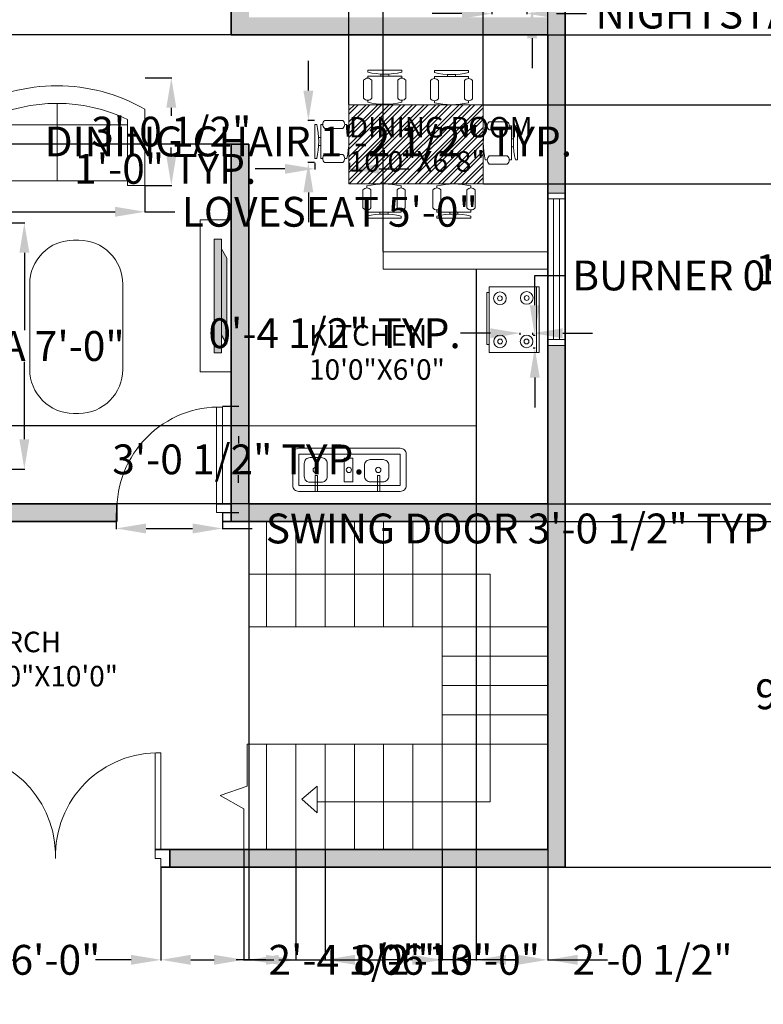
# Model space of a CAD drawing. Units: inches. Extents: x 1294 to 2470, y 659 to 1389.
# Tile 2 of 4: x 1460 to 1714, y 695 to 1031. Entities that reach past the tile are written whole.
import ezdxf

# ---------------------------------------------------------------- set-up
doc = ezdxf.new("R2010")
doc.units = ezdxf.units.IN
doc.header["$MEASUREMENT"] = 0
for name, color, linetype, lineweight in [('A-ANNO-DIMS', 2, 'Continuous', 18), ('A-AREA-IDEN', 7, 'Continuous', 20), ('A-DOOR', 3, 'Continuous', 18), ('A-EQPM', 8, 'Continuous', 18), ('A-FLOR-CASE', 9, 'Continuous', 20), ('A-FLOR-FIXT', 9, 'Continuous', 18), ('A-FLOR-STRS', 7, 'Continuous', 20), ('A-FURN', 8, 'Continuous', 18), ('A-FURN-PATT', 9, 'Continuous', 13), ('A-GLAZ', 4, 'Continuous', 18), ('A-WALL', 7, 'Continuous', 35), ('A-WALL-PATT', 252, 'Continuous', 13)]:
    doc.layers.add(name, color=color, linetype=linetype, lineweight=lineweight)
doc.styles.get("Standard").update_dxf_attribs({"font": 'arial.ttf'})
doc.dimstyles.get("Standard").update_dxf_attribs({"dimtxt": 10.18, "dimasz": 10.18, "dimexe": 0.18, "dimexo": 0.0625, "dimgap": 0.09, "dimtad": 0, "dimtih": 1, "dimtoh": 1, "dimdec": 0, "dimzin": 0, "dimdsep": 46, "dimlunit": 3, "dimtxsty": 'Standard', "dimcen": 0.09, "dimadec": 0, "dimazin": 0, "dimtfac": 1, "dimtdec": 0, "dimtofl": 0, "dimtmove": 0, "dimatfit": 3, "dimfxl": 1, "dimtolj": 1, "dimtzin": 0, "dimarcsym": 0})

# ---------------------------------------------------------------- blocks, each defined once
blk = doc.blocks.new('Sofa - Roundback Loveseat 5 ft.')
for p, q in [((0, -32.44198), (0, -5.99998)), ((-24, -33.99998), (-24, -11.46958)), ((-23.9998, -13.38178), (23.99986, -13.38178)), ((24.00004, -33.99998), (24.00004, -11.46958)), ((-24, -32.44198), (24.00004, -32.44198))]:
    blk.add_line(p, q)
for points in [[(-24, -33.99998), (-30, -33.99998), (-30, -7.99998)], [(30.00004, -7.99998), (30.00004, -33.99998), (24.00004, -33.99998)]]:
    blk.add_lwpolyline(points)
for centre, radius, start, end in [((0, -60.24998), 60.24998, 60.13715, 119.8628), ((0, -61.38438), 55.38444, 64.32083, 115.6792)]:
    blk.add_arc(centre, radius, start, end)
blk = doc.blocks.new('Chair - Desk')
for p, q in [((-8.5, 0), (-8.5, -1)), ((-8.5, 0), (8.5, 0)), ((8.5, 0), (8.5, -1)), ((-8.5, -3), (-8.5, -4)), ((-8.5, -3), (8.5, -3)), ((-2, -3), (-2, -1.9355)), ((2, -1.9576), (2, -3)), ((8.5, -3), (8.5, -4)), ((-10.5, -5), (-10.5, -14)), ((-6.5, -14), (-6.5, -5)), ((6.5, -5), (6.5, -14)), ((10.5, -14), (10.5, -5)), ((-8.5, -15), (-8.5, -16)), ((8.5, -15), (8.5, -16))]:
    blk.add_line(p, q)
for centre, radius, start, end in [((-8.5, -6.5), 2.5, 36.8699, 143.1301), ((0, 34.625), 36.625, 256.5803, 283.4197), ((8.5, -6.5), 2.5, 36.8699, 143.1301), ((-8.5, -12.5), 2.5, 216.8699, 323.1301), ((8.5, -12.5), 2.5, 216.8699, 323.1301), ((0, 19.625), 36.625, 256.5803, 283.4197)]:
    blk.add_arc(centre, radius, start, end)
blk = doc.blocks.new('DOOR-SWING-36')
for p, q in [((34.01, 0), (34.01, 36)), ((36.01, 3), (36.01, 36)), ((34.01, 0), (36.01, 0))]:
    blk.add_line(p, q)
blk.add_arc((35.01, 1), 35.01, 88.3634, 181.6366)
blk = doc.blocks.new('WIN-48')
for p, q in [((0, 6), (0, 0)), ((2, 6), (2, 0)), ((50, 4), (2, 4)), ((50, 6), (50, 0)), ((52, 6), (52, 0)), ((50, 2), (2, 2))]:
    blk.add_line(p, q)
blk = doc.blocks.new('COOKTOP-BURNER')
for radius in [2.16, 2.16, 0.819]:
    blk.add_circle((2.16, 2.16), radius)
blk = doc.blocks.new('*D14')
at = {"layer": 'A-ANNO-DIMS', "color": 0, "lineweight": -2, "transparency": 16777216}
for p, q in [((1558.97, 1006.76), (1558.97, 1016.94)), ((1561.07, 996.58), (1558.79, 996.58)), ((1561.07, 982.2), (1558.79, 982.2)), ((1558.97, 972.02), (1558.97, 961.84))]:
    blk.add_line(p, q, dxfattribs=at)
at = {"layer": 'A-ANNO-DIMS', "color": 0, "transparency": 16777216}
for points in [[(1557.27, 1006.76), (1560.67, 1006.76), (1558.97, 996.58)], [(1557.27, 972.02), (1560.67, 972.02), (1558.97, 982.2)]]:
    blk.add_solid(points, dxfattribs=at)
at = {"layer": 'Defpoints', "color": 0, "transparency": 16777216}
for p in [(1558.97, 996.58), (1561.13, 996.58), (1561.13, 982.2)]:
    blk.add_point(p, dxfattribs=at)
at = {"layer": 'A-ANNO-DIMS', "color": 0, "transparency": 16777216, "insert": (1558.97, 989.39), "char_height": 10.18, "attachment_point": 5}
blk.add_mtext('\\A1;DINING CHAIR 1\'-2 1/2" TYP.', dxfattribs=at)
blk = doc.blocks.new('*D15')
at = {"layer": 'A-ANNO-DIMS', "color": 0, "lineweight": -2, "transparency": 16777216}
for p, q in [((1561.13, 982.13), (1561.13, 979.86)), ((1573, 982.13), (1573, 979.86)), ((1550.95, 980.04), (1540.77, 980.04)), ((1583.18, 980.04), (1593.36, 980.04))]:
    blk.add_line(p, q, dxfattribs=at)
at = {"layer": 'A-ANNO-DIMS', "color": 0, "transparency": 16777216}
for points in [[(1550.95, 981.74), (1550.95, 978.34), (1561.13, 980.04)], [(1583.18, 981.74), (1583.18, 978.34), (1573, 980.04)]]:
    blk.add_solid(points, dxfattribs=at)
at = {"layer": 'Defpoints', "color": 0, "transparency": 16777216}
for p in [(1561.13, 982.2), (1573, 982.2), (1561.13, 980.04)]:
    blk.add_point(p, dxfattribs=at)
at = {"layer": 'A-ANNO-DIMS', "color": 0, "transparency": 16777216, "insert": (1510.13, 980.04), "char_height": 10.18, "attachment_point": 5}
blk.add_mtext('\\A1;1\'-0" TYP.', dxfattribs=at)
blk = doc.blocks.new('*D16')
at = {"layer": 'A-ANNO-DIMS', "color": 0, "lineweight": -2, "transparency": 16777216}
for p, q in [((1493.39, 862.72), (1493.39, 857.16)), ((1529.66, 862.72), (1529.66, 857.16)), ((1503.57, 857.34), (1519.48, 857.34)), ((1529.66, 857.34), (1539.84, 857.34))]:
    blk.add_line(p, q, dxfattribs=at)
at = {"layer": 'A-ANNO-DIMS', "color": 0, "transparency": 16777216}
for points in [[(1503.57, 859.04), (1503.57, 855.65), (1493.39, 857.34)], [(1519.48, 859.04), (1519.48, 855.65), (1529.66, 857.34)]]:
    blk.add_solid(points, dxfattribs=at)
at = {"layer": 'Defpoints', "color": 0, "transparency": 16777216}
for p in [(1493.39, 862.78), (1529.66, 862.78), (1529.66, 857.34)]:
    blk.add_point(p, dxfattribs=at)
at = {"layer": 'A-ANNO-DIMS', "color": 0, "transparency": 16777216, "insert": (1632.17, 857.34), "char_height": 10.18, "attachment_point": 5}
blk.add_mtext('\\A1;SWING DOOR 3\'-0 1/2" TYP.', dxfattribs=at)
blk = doc.blocks.new('*D17')
at = {"layer": 'A-ANNO-DIMS', "color": 0, "lineweight": -2, "transparency": 16777216}
for p, q in [((1529.72, 899.06), (1535.28, 899.06)), ((1535.1, 888.88), (1535.1, 886.28)), ((1535.1, 872.96), (1535.1, 875.56)), ((1529.72, 862.78), (1535.28, 862.78))]:
    blk.add_line(p, q, dxfattribs=at)
at = {"layer": 'A-ANNO-DIMS', "color": 0, "transparency": 16777216}
for points in [[(1533.41, 888.88), (1536.8, 888.88), (1535.1, 899.06)], [(1533.41, 872.96), (1536.8, 872.96), (1535.1, 862.78)]]:
    blk.add_solid(points, dxfattribs=at)
at = {"layer": 'Defpoints', "color": 0, "transparency": 16777216}
for p in [(1529.66, 899.06), (1535.1, 899.06), (1529.66, 862.78)]:
    blk.add_point(p, dxfattribs=at)
at = {"layer": 'A-ANNO-DIMS', "color": 0, "transparency": 16777216, "insert": (1535.1, 880.92), "char_height": 10.18, "attachment_point": 5}
blk.add_mtext('\\A1;3\'-0 1/2" TYP.', dxfattribs=at)
blk = doc.blocks.new('*D22')
at = {"layer": 'A-ANNO-DIMS', "color": 0, "lineweight": -2, "transparency": 16777216}
for p, q in [((1636.23, 933.49), (1636.23, 943.67)), ((1636.23, 943.67), (1646.41, 943.67)), ((1635.64, 923.31), (1636.41, 923.31)), ((1635.64, 918.98), (1636.41, 918.98)), ((1636.23, 908.8), (1636.23, 898.62))]:
    blk.add_line(p, q, dxfattribs=at)
at = {"layer": 'A-ANNO-DIMS', "color": 0, "transparency": 16777216}
for points in [[(1634.53, 933.49), (1637.92, 933.49), (1636.23, 923.31)], [(1634.53, 908.8), (1637.92, 908.8), (1636.23, 918.98)]]:
    blk.add_solid(points, dxfattribs=at)
at = {"layer": 'Defpoints', "color": 0, "transparency": 16777216}
for p in [(1635.58, 923.31), (1636.23, 923.31), (1635.58, 918.98)]:
    blk.add_point(p, dxfattribs=at)
at = {"layer": 'A-ANNO-DIMS', "color": 0, "transparency": 16777216, "insert": (1721.16, 943.67), "char_height": 10.18, "attachment_point": 5}
blk.add_mtext('\\A1;BURNER 0\'-4 1/2" TYP.', dxfattribs=at)
blk = doc.blocks.new('*D23')
at = {"layer": 'A-ANNO-DIMS', "color": 0, "lineweight": -2, "transparency": 16777216}
for p, q in [((1621.07, 923.96), (1610.89, 923.96)), ((1631.25, 923.37), (1631.25, 924.14)), ((1635.58, 923.37), (1635.58, 924.14)), ((1645.76, 923.96), (1655.94, 923.96))]:
    blk.add_line(p, q, dxfattribs=at)
at = {"layer": 'A-ANNO-DIMS', "color": 0, "transparency": 16777216}
for points in [[(1621.07, 925.65), (1621.07, 922.26), (1631.25, 923.96)], [(1645.76, 925.65), (1645.76, 922.26), (1635.58, 923.96)]]:
    blk.add_solid(points, dxfattribs=at)
at = {"layer": 'Defpoints', "color": 0, "transparency": 16777216}
for p in [(1631.25, 923.96), (1631.25, 923.31), (1635.58, 923.31)]:
    blk.add_point(p, dxfattribs=at)
at = {"layer": 'A-ANNO-DIMS', "color": 0, "transparency": 16777216, "insert": (1567.91, 923.96), "char_height": 10.18, "attachment_point": 5}
blk.add_mtext('\\A1;0\'-4 1/2" TYP.', dxfattribs=at)
blk = doc.blocks.new('*D26')
at = {"layer": 'A-ANNO-DIMS', "color": 0, "lineweight": -2, "transparency": 16777216}
for p, q in [((1621.57, 1034.72), (1621.57, 1032.82)), ((1633.51, 1034.72), (1633.51, 1032.82)), ((1611.39, 1033), (1601.21, 1033)), ((1643.69, 1033), (1653.87, 1033))]:
    blk.add_line(p, q, dxfattribs=at)
at = {"layer": 'A-ANNO-DIMS', "color": 0, "transparency": 16777216}
for points in [[(1611.39, 1034.69), (1611.39, 1031.3), (1621.57, 1033)], [(1643.69, 1034.69), (1643.69, 1031.3), (1633.51, 1033)]]:
    blk.add_solid(points, dxfattribs=at)
at = {"layer": 'Defpoints', "color": 0, "transparency": 16777216}
for p in [(1621.57, 1034.79), (1633.51, 1034.79), (1633.51, 1033)]:
    blk.add_point(p, dxfattribs=at)
at = {"layer": 'A-ANNO-DIMS', "color": 0, "transparency": 16777216, "insert": (1732.93, 1033), "char_height": 10.18, "attachment_point": 5}
blk.add_mtext('\\A1;NIGHTSTAND 1\'-0" TYP.', dxfattribs=at)
blk = doc.blocks.new('*D27')
at = {"layer": 'A-ANNO-DIMS', "color": 0, "lineweight": -2, "transparency": 16777216}
for p, q in [((1635.3, 1055.87), (1635.3, 1066.05)), ((1633.57, 1045.69), (1635.48, 1045.69)), ((1633.57, 1034.79), (1635.48, 1034.79)), ((1635.3, 1024.61), (1635.3, 1014.43))]:
    blk.add_line(p, q, dxfattribs=at)
at = {"layer": 'A-ANNO-DIMS', "color": 0, "transparency": 16777216}
for points in [[(1633.6, 1055.87), (1637, 1055.87), (1635.3, 1045.69)], [(1633.6, 1024.61), (1637, 1024.61), (1635.3, 1034.79)]]:
    blk.add_solid(points, dxfattribs=at)
at = {"layer": 'Defpoints', "color": 0, "transparency": 16777216}
for p in [(1633.51, 1045.69), (1635.3, 1045.69), (1633.51, 1034.79)]:
    blk.add_point(p, dxfattribs=at)
at = {"layer": 'A-ANNO-DIMS', "color": 0, "transparency": 16777216, "insert": (1635.3, 1040.24), "char_height": 10.18, "attachment_point": 5}
blk.add_mtext('\\A1;0\'-11" TYP.', dxfattribs=at)
blk = doc.blocks.new('*D28')
at = {"layer": 'A-ANNO-DIMS', "color": 0, "lineweight": -2, "transparency": 16777216}
for p, q in [((1449.5, 961.6), (1462.22, 961.6)), ((1462.04, 951.42), (1462.04, 924.95)), ((1462.04, 887.78), (1462.04, 914.24)), ((1449.5, 877.6), (1462.22, 877.6))]:
    blk.add_line(p, q, dxfattribs=at)
at = {"layer": 'A-ANNO-DIMS', "color": 0, "transparency": 16777216}
for points in [[(1460.34, 951.42), (1463.74, 951.42), (1462.04, 961.6)], [(1460.34, 887.78), (1463.74, 887.78), (1462.04, 877.6)]]:
    blk.add_solid(points, dxfattribs=at)
at = {"layer": 'Defpoints', "color": 0, "transparency": 16777216}
for p in [(1449.44, 961.6), (1462.04, 961.6), (1449.44, 877.6)]:
    blk.add_point(p, dxfattribs=at)
at = {"layer": 'A-ANNO-DIMS', "color": 0, "transparency": 16777216, "insert": (1462.04, 919.6), "char_height": 10.18, "attachment_point": 5}
blk.add_mtext('\\A1;SOFA 7\'-0"', dxfattribs=at)
blk = doc.blocks.new('*D30')
at = {"layer": 'A-ANNO-DIMS', "color": 0, "lineweight": -2, "transparency": 16777216}
for p, q in [((1443.19, 974.33), (1443.19, 965.21)), ((1503.19, 974.33), (1503.19, 965.21)), ((1453.37, 965.39), (1493.01, 965.39)), ((1503.19, 965.39), (1513.37, 965.39))]:
    blk.add_line(p, q, dxfattribs=at)
at = {"layer": 'A-ANNO-DIMS', "color": 0, "transparency": 16777216}
for points in [[(1453.37, 967.09), (1453.37, 963.7), (1443.19, 965.39)], [(1493.01, 967.09), (1493.01, 963.7), (1503.19, 965.39)]]:
    blk.add_solid(points, dxfattribs=at)
at = {"layer": 'Defpoints', "color": 0, "transparency": 16777216}
for p in [(1443.19, 974.39), (1503.19, 974.39), (1503.19, 965.39)]:
    blk.add_point(p, dxfattribs=at)
at = {"layer": 'A-ANNO-DIMS', "color": 0, "transparency": 16777216, "insert": (1566.29, 965.39), "char_height": 10.18, "attachment_point": 5}
blk.add_mtext('\\A1;LOVESEAT 5\'-0"', dxfattribs=at)
blk = doc.blocks.new('*D31')
at = {"layer": 'A-ANNO-DIMS', "color": 0, "lineweight": -2, "transparency": 16777216}
for p, q in [((1503.26, 1011.06), (1512.37, 1011.06)), ((1512.19, 1000.88), (1512.19, 998.09)), ((1512.19, 984.57), (1512.19, 987.37)), ((1503.26, 974.39), (1512.37, 974.39))]:
    blk.add_line(p, q, dxfattribs=at)
at = {"layer": 'A-ANNO-DIMS', "color": 0, "transparency": 16777216}
for points in [[(1510.5, 1000.88), (1513.89, 1000.88), (1512.19, 1011.06)], [(1510.5, 984.57), (1513.89, 984.57), (1512.19, 974.39)]]:
    blk.add_solid(points, dxfattribs=at)
at = {"layer": 'Defpoints', "color": 0, "transparency": 16777216}
for p in [(1503.19, 1011.06), (1512.19, 1011.06), (1503.19, 974.39)]:
    blk.add_point(p, dxfattribs=at)
at = {"layer": 'A-ANNO-DIMS', "color": 0, "transparency": 16777216, "insert": (1512.19, 992.73), "char_height": 10.18, "attachment_point": 5}
blk.add_mtext('\\A1;3\'-0 1/2"', dxfattribs=at)
blk = doc.blocks.new('*D32')
at = {"layer": 'A-ANNO-DIMS', "color": 0, "lineweight": -2, "transparency": 16777216}
for p, q in [((1554.66, 747.72), (1554.66, 710)), ((1564.66, 747.72), (1564.66, 710)), ((1544.48, 710.18), (1534.3, 710.18)), ((1574.84, 710.18), (1585.02, 710.18))]:
    blk.add_line(p, q, dxfattribs=at)
at = {"layer": 'A-ANNO-DIMS', "color": 0, "transparency": 16777216}
for points in [[(1544.48, 711.88), (1544.48, 708.49), (1554.66, 710.18)], [(1574.84, 711.88), (1574.84, 708.49), (1564.66, 710.18)]]:
    blk.add_solid(points, dxfattribs=at)
at = {"layer": 'Defpoints', "color": 0, "transparency": 16777216}
for p in [(1554.66, 747.78), (1564.66, 747.78), (1564.66, 710.18)]:
    blk.add_point(p, dxfattribs=at)
at = {"layer": 'A-ANNO-DIMS', "color": 0, "transparency": 16777216, "insert": (1602.6, 710.18), "char_height": 10.18, "attachment_point": 5}
blk.add_mtext('\\A1;0\'-10"', dxfattribs=at)
blk = doc.blocks.new('*D33')
at = {"layer": 'A-ANNO-DIMS', "color": 0, "lineweight": -2, "transparency": 16777216}
for p, q in [((1604.66, 747.72), (1604.66, 710)), ((1640.66, 747.72), (1640.66, 710)), ((1594.48, 710.18), (1584.3, 710.18)), ((1650.84, 710.18), (1661.02, 710.18))]:
    blk.add_line(p, q, dxfattribs=at)
at = {"layer": 'A-ANNO-DIMS', "color": 0, "transparency": 16777216}
for points in [[(1594.48, 711.88), (1594.48, 708.49), (1604.66, 710.18)], [(1650.84, 711.88), (1650.84, 708.49), (1640.66, 710.18)]]:
    blk.add_solid(points, dxfattribs=at)
at = {"layer": 'Defpoints', "color": 0, "transparency": 16777216}
for p in [(1604.66, 747.78), (1640.66, 747.78), (1640.66, 710.18)]:
    blk.add_point(p, dxfattribs=at)
at = {"layer": 'A-ANNO-DIMS', "color": 0, "transparency": 16777216, "insert": (1622.66, 710.18), "char_height": 10.18, "attachment_point": 5}
blk.add_mtext('\\A1;3\'-0"', dxfattribs=at)
blk = doc.blocks.new('*D34')
at = {"layer": 'A-ANNO-DIMS', "color": 0, "lineweight": -2, "transparency": 16777216}
for p, q in [((1436.66, 741.72), (1436.66, 710)), ((1508.66, 741.72), (1508.66, 710)), ((1446.84, 710.18), (1459.01, 710.18)), ((1498.48, 710.18), (1486.31, 710.18))]:
    blk.add_line(p, q, dxfattribs=at)
at = {"layer": 'A-ANNO-DIMS', "color": 0, "transparency": 16777216}
for points in [[(1446.84, 711.88), (1446.84, 708.49), (1436.66, 710.18)], [(1498.48, 711.88), (1498.48, 708.49), (1508.66, 710.18)]]:
    blk.add_solid(points, dxfattribs=at)
at = {"layer": 'Defpoints', "color": 0, "transparency": 16777216}
for p in [(1436.66, 741.78), (1508.66, 741.78), (1508.66, 710.18)]:
    blk.add_point(p, dxfattribs=at)
at = {"layer": 'A-ANNO-DIMS', "color": 0, "transparency": 16777216, "insert": (1472.66, 710.18), "char_height": 10.18, "attachment_point": 5}
blk.add_mtext('\\A1;6\'-0"', dxfattribs=at)
blk = doc.blocks.new('*D36')
at = {"layer": 'A-ANNO-DIMS', "color": 0, "lineweight": -2, "transparency": 16777216}
for p, q in [((1536.95, 747.72), (1536.95, 710)), ((1508.66, 741.72), (1508.66, 710)), ((1518.84, 710.18), (1526.77, 710.18)), ((1536.95, 710.18), (1547.13, 710.18))]:
    blk.add_line(p, q, dxfattribs=at)
at = {"layer": 'A-ANNO-DIMS', "color": 0, "transparency": 16777216}
for points in [[(1518.84, 711.88), (1518.84, 708.49), (1508.66, 710.18)], [(1526.77, 711.88), (1526.77, 708.49), (1536.95, 710.18)]]:
    blk.add_solid(points, dxfattribs=at)
at = {"layer": 'Defpoints', "color": 0, "transparency": 16777216}
for p in [(1536.95, 747.78), (1508.66, 741.78), (1536.95, 710.18)]:
    blk.add_point(p, dxfattribs=at)
at = {"layer": 'A-ANNO-DIMS', "color": 0, "transparency": 16777216, "insert": (1572.69, 710.18), "char_height": 10.18, "attachment_point": 5}
blk.add_mtext('\\A1;2\'-4 1/2"', dxfattribs=at)
blk = doc.blocks.new('*D37')
at = {"layer": 'A-ANNO-DIMS', "color": 0, "lineweight": -2, "transparency": 16777216}
for p, q in [((1640.72, 859.78), (1730.86, 859.78)), ((1730.68, 849.6), (1730.68, 806.07)), ((1730.68, 751.96), (1730.68, 795.5)), ((1646.72, 741.78), (1730.86, 741.78))]:
    blk.add_line(p, q, dxfattribs=at)
at = {"layer": 'A-ANNO-DIMS', "color": 0, "transparency": 16777216}
for points in [[(1728.99, 849.6), (1732.38, 849.6), (1730.68, 859.78)], [(1728.99, 751.96), (1732.38, 751.96), (1730.68, 741.78)]]:
    blk.add_solid(points, dxfattribs=at)
at = {"layer": 'Defpoints', "color": 0, "transparency": 16777216}
for p in [(1640.66, 859.78), (1730.68, 859.78), (1646.66, 741.78)]:
    blk.add_point(p, dxfattribs=at)
at = {"layer": 'A-ANNO-DIMS', "color": 0, "transparency": 16777216, "insert": (1730.68, 800.78), "char_height": 10.18, "attachment_point": 5}
blk.add_mtext('\\A1;9\'-10"', dxfattribs=at)
blk = doc.blocks.new('*D38')
at = {"layer": 'A-ANNO-DIMS', "color": 0, "lineweight": -2, "transparency": 16777216}
for p, q in [((1640.72, 1025.78), (1730.86, 1025.78)), ((1730.68, 1015.6), (1730.68, 951.07)), ((1730.68, 875.96), (1730.68, 940.49)), ((1640.72, 865.78), (1730.86, 865.78))]:
    blk.add_line(p, q, dxfattribs=at)
at = {"layer": 'A-ANNO-DIMS', "color": 0, "transparency": 16777216}
for points in [[(1728.99, 1015.6), (1732.38, 1015.6), (1730.68, 1025.78)], [(1728.99, 875.96), (1732.38, 875.96), (1730.68, 865.78)]]:
    blk.add_solid(points, dxfattribs=at)
at = {"layer": 'Defpoints', "color": 0, "transparency": 16777216}
for p in [(1640.66, 1025.78), (1730.68, 1025.78), (1640.66, 865.78)]:
    blk.add_point(p, dxfattribs=at)
at = {"layer": 'A-ANNO-DIMS', "color": 0, "transparency": 16777216, "insert": (1730.68, 945.78), "char_height": 10.18, "attachment_point": 5}
blk.add_mtext('\\A1;13\'-4"', dxfattribs=at)
blk = doc.blocks.new('*D39')
at = {"layer": 'A-ANNO-DIMS', "color": 0, "lineweight": -2, "transparency": 16777216}
for p, q in [((1640.72, 1147.78), (1730.86, 1147.78)), ((1730.68, 1137.6), (1730.68, 1092.07)), ((1730.68, 1035.96), (1730.68, 1081.5)), ((1640.72, 1025.78), (1730.86, 1025.78))]:
    blk.add_line(p, q, dxfattribs=at)
at = {"layer": 'A-ANNO-DIMS', "color": 0, "transparency": 16777216}
for points in [[(1728.99, 1137.6), (1732.38, 1137.6), (1730.68, 1147.78)], [(1728.99, 1035.96), (1732.38, 1035.96), (1730.68, 1025.78)]]:
    blk.add_solid(points, dxfattribs=at)
at = {"layer": 'Defpoints', "color": 0, "transparency": 16777216}
for p in [(1640.66, 1147.78), (1730.68, 1147.78), (1640.66, 1025.78)]:
    blk.add_point(p, dxfattribs=at)
at = {"layer": 'A-ANNO-DIMS', "color": 0, "transparency": 16777216, "insert": (1730.68, 1086.78), "char_height": 10.18, "attachment_point": 5}
blk.add_mtext('\\A1;10\'-2"', dxfattribs=at)
blk = doc.blocks.new('*D47')
at = {"layer": 'A-ANNO-DIMS', "color": 0, "lineweight": -2, "transparency": 16777216}
for p, q in [((1532.6, 1025.78), (1320.88, 1025.78)), ((1321.06, 1015.6), (1321.06, 1012.46)), ((1321.06, 998.59), (1321.06, 1001.74)), ((1538.6, 988.41), (1320.88, 988.41))]:
    blk.add_line(p, q, dxfattribs=at)
at = {"layer": 'A-ANNO-DIMS', "color": 0, "transparency": 16777216}
for points in [[(1319.37, 1015.6), (1322.76, 1015.6), (1321.06, 1025.78)], [(1319.37, 998.59), (1322.76, 998.59), (1321.06, 988.41)]]:
    blk.add_solid(points, dxfattribs=at)
at = {"layer": 'Defpoints', "color": 0, "transparency": 16777216}
for p in [(1321.06, 1025.78), (1532.66, 1025.78), (1538.66, 988.41)]:
    blk.add_point(p, dxfattribs=at)
at = {"layer": 'A-ANNO-DIMS', "color": 0, "transparency": 16777216, "insert": (1321.06, 1007.1), "char_height": 10.18, "attachment_point": 5}
blk.add_mtext('\\A1;3\'-1 1/2"', dxfattribs=at)
blk = doc.blocks.new('*D48')
at = {"layer": 'A-ANNO-DIMS', "color": 0, "lineweight": -2, "transparency": 16777216}
for p, q in [((1538.66, 865.72), (1538.66, 710)), ((1640.66, 865.72), (1640.66, 710)), ((1548.84, 710.18), (1576.03, 710.18)), ((1630.48, 710.18), (1603.29, 710.18))]:
    blk.add_line(p, q, dxfattribs=at)
at = {"layer": 'A-ANNO-DIMS', "color": 0, "transparency": 16777216}
for points in [[(1548.84, 711.88), (1548.84, 708.49), (1538.66, 710.18)], [(1630.48, 711.88), (1630.48, 708.49), (1640.66, 710.18)]]:
    blk.add_solid(points, dxfattribs=at)
at = {"layer": 'Defpoints', "color": 0, "transparency": 16777216}
for p in [(1538.66, 865.78), (1640.66, 865.78), (1640.66, 710.18)]:
    blk.add_point(p, dxfattribs=at)
at = {"layer": 'A-ANNO-DIMS', "color": 0, "transparency": 16777216, "insert": (1589.66, 710.18), "char_height": 10.18, "attachment_point": 5}
blk.add_mtext('\\A1;8\'-6"', dxfattribs=at)
blk = doc.blocks.new('*D49')
at = {"layer": 'A-ANNO-DIMS', "color": 0, "lineweight": -2, "transparency": 16777216}
for p, q in [((1616.19, 945.72), (1616.19, 710)), ((1640.66, 945.72), (1640.66, 710)), ((1626.37, 710.18), (1630.48, 710.18)), ((1640.66, 710.18), (1650.84, 710.18))]:
    blk.add_line(p, q, dxfattribs=at)
at = {"layer": 'A-ANNO-DIMS', "color": 0, "transparency": 16777216}
for points in [[(1626.37, 711.88), (1626.37, 708.49), (1616.19, 710.18)], [(1630.48, 711.88), (1630.48, 708.49), (1640.66, 710.18)]]:
    blk.add_solid(points, dxfattribs=at)
at = {"layer": 'Defpoints', "color": 0, "transparency": 16777216}
for p in [(1616.19, 945.78), (1640.66, 945.78), (1640.66, 710.18)]:
    blk.add_point(p, dxfattribs=at)
at = {"layer": 'A-ANNO-DIMS', "color": 0, "transparency": 16777216, "insert": (1676.41, 710.18), "char_height": 10.18, "attachment_point": 5}
blk.add_mtext('\\A1;2\'-0 1/2"', dxfattribs=at)
blk = doc.blocks.new('*D50')
at = {"layer": 'A-ANNO-DIMS', "color": 0, "lineweight": -2, "transparency": 16777216}
for p, q in [((1562.59, 1373.38), (1552.41, 1373.38)), ((1572.77, 1001.97), (1572.77, 1373.56)), ((1618.65, 1001.97), (1618.65, 1373.56)), ((1628.83, 1373.38), (1639.01, 1373.38))]:
    blk.add_line(p, q, dxfattribs=at)
at = {"layer": 'A-ANNO-DIMS', "color": 0, "transparency": 16777216}
for points in [[(1562.59, 1375.08), (1562.59, 1371.69), (1572.77, 1373.38)], [(1628.83, 1375.08), (1628.83, 1371.69), (1618.65, 1373.38)]]:
    blk.add_solid(points, dxfattribs=at)
at = {"layer": 'Defpoints', "color": 0, "transparency": 16777216}
for p in [(1618.65, 1373.38), (1572.77, 1001.91), (1618.65, 1001.91)]:
    blk.add_point(p, dxfattribs=at)
at = {"layer": 'A-ANNO-DIMS', "color": 0, "transparency": 16777216, "insert": (1595.71, 1373.38), "char_height": 10.18, "attachment_point": 5}
blk.add_mtext('\\A1;3\'-10"', dxfattribs=at)
blk = doc.blocks.new('*D51')
at = {"layer": 'A-ANNO-DIMS', "color": 0, "lineweight": -2, "transparency": 16777216}
for p, q in [((1730.68, 1001.91), (1730.68, 1012.09)), ((1730.68, 1012.09), (1740.86, 1012.09)), ((1618.71, 1001.91), (1730.86, 1001.91)), ((1730.68, 985.08), (1730.68, 991.73)), ((1618.71, 974.9), (1730.86, 974.9))]:
    blk.add_line(p, q, dxfattribs=at)
at = {"layer": 'A-ANNO-DIMS', "color": 0, "transparency": 16777216}
for points in [[(1728.99, 991.73), (1732.38, 991.73), (1730.68, 1001.91)], [(1728.99, 985.08), (1732.38, 985.08), (1730.68, 974.9)]]:
    blk.add_solid(points, dxfattribs=at)
at = {"layer": 'Defpoints', "color": 0, "transparency": 16777216}
for p in [(1618.65, 1001.91), (1730.68, 1001.91), (1618.65, 974.9)]:
    blk.add_point(p, dxfattribs=at)
at = {"layer": 'A-ANNO-DIMS', "color": 0, "transparency": 16777216, "insert": (1754.57, 1012.09), "char_height": 10.18, "attachment_point": 5}
blk.add_mtext('\\A1;2\'-3"', dxfattribs=at)
blk = doc.blocks.new('*D52')
at = {"layer": 'A-ANNO-DIMS', "color": 0, "lineweight": -2, "transparency": 16777216}
for p, q in [((1321.06, 892.37), (1321.06, 902.55)), ((1321.06, 902.55), (1331.24, 902.55)), ((1538.6, 892.37), (1320.88, 892.37)), ((1321.06, 875.96), (1321.06, 882.19)), ((1538.6, 865.78), (1320.88, 865.78))]:
    blk.add_line(p, q, dxfattribs=at)
at = {"layer": 'A-ANNO-DIMS', "color": 0, "transparency": 16777216}
for points in [[(1319.37, 882.19), (1322.76, 882.19), (1321.06, 892.37)], [(1319.37, 875.96), (1322.76, 875.96), (1321.06, 865.78)]]:
    blk.add_solid(points, dxfattribs=at)
at = {"layer": 'Defpoints', "color": 0, "transparency": 16777216}
for p in [(1321.06, 892.37), (1538.66, 892.37), (1538.66, 865.78)]:
    blk.add_point(p, dxfattribs=at)
at = {"layer": 'A-ANNO-DIMS', "color": 0, "transparency": 16777216, "insert": (1356.81, 902.55), "char_height": 10.18, "attachment_point": 5}
blk.add_mtext('\\A1;2\'-2 1/2"', dxfattribs=at)
blk = doc.blocks.new('*D53')
at = {"layer": 'A-ANNO-DIMS', "color": 0, "lineweight": -2, "transparency": 16777216}
for p, q in [((1584.52, 951.85), (1584.52, 1373.56)), ((1594.7, 1373.38), (1598.77, 1373.38)), ((1630.48, 1373.38), (1626.42, 1373.38)), ((1640.66, 951.85), (1640.66, 1373.56))]:
    blk.add_line(p, q, dxfattribs=at)
at = {"layer": 'A-ANNO-DIMS', "color": 0, "transparency": 16777216}
for points in [[(1594.7, 1375.08), (1594.7, 1371.69), (1584.52, 1373.38)], [(1630.48, 1375.08), (1630.48, 1371.69), (1640.66, 1373.38)]]:
    blk.add_solid(points, dxfattribs=at)
at = {"layer": 'Defpoints', "color": 0, "transparency": 16777216}
for p in [(1640.66, 1373.38), (1584.52, 951.78), (1640.66, 951.78)]:
    blk.add_point(p, dxfattribs=at)
at = {"layer": 'A-ANNO-DIMS', "color": 0, "transparency": 16777216, "insert": (1612.59, 1373.38), "char_height": 10.18, "attachment_point": 5}
blk.add_mtext('\\A1;4\'-8"', dxfattribs=at)

msp = doc.modelspace()

# ---------------------------------------------------------------- hatches: boundary and pattern name
at = {"layer": 'A-FURN-PATT'}
h = msp.add_hatch(dxfattribs=at)
h.set_pattern_fill('ANSI32', color=256, scale=7.5)
h.paths.add_polyline_path([(1618.65, 1001.91), (1572.77, 1001.91), (1572.77, 974.9), (1618.65, 974.9)])
h = msp.add_hatch(color=256, dxfattribs=at)
h.dxf.hatch_style = 1
h.paths.add_polyline_path([(1531.14, 949.56), (1529.27, 952.78), (1529.27, 923.33), (1531.14, 920.22)])
h.paths.add_polyline_path([(1526.84, 917.31), (1529.27, 917.31), (1529.27, 956.06), (1526.84, 956.06)])
at = {"layer": 'A-WALL-PATT'}
h = msp.add_hatch(color=256, dxfattribs=at)
h.dxf.hatch_style = 1
h.paths.add_polyline_path([(1412.66, 1335.78), (1446.66, 1335.78), (1446.66, 1341.78), (1406.66, 1341.78), (1406.66, 1197.78), (1412.66, 1197.78), (1412.66, 1213.78), (1480.66, 1213.78), (1480.66, 1186.78), (1481.11, 1186.78, -0.021978), (1483.66, 1186.78), (1486.66, 1186.78), (1486.66, 1213.78), (1493.66, 1213.78), (1493.66, 1216.78, -0.014283), (1493.66, 1218.78), (1493.66, 1219.78), (1412.66, 1219.78)])
h.paths.add_polyline_path([(1563.66, 1341.78), (1498.66, 1341.78), (1498.66, 1335.78), (1532.66, 1335.78), (1532.66, 1219.78), (1532.66, 1213.78), (1538.66, 1213.78), (1538.66, 1219.78), (1538.66, 1335.78), (1563.66, 1335.78)])
h.paths.add_polyline_path([(1646.66, 1341.78), (1615.66, 1341.78), (1615.66, 1335.78), (1640.66, 1335.78), (1640.66, 1219.78), (1622.13, 1219.78), (1622.13, 1216.78, -0.017236), (1622.13, 1214.78), (1622.13, 1213.78), (1640.66, 1213.78), (1640.66, 1197.78), (1646.66, 1197.78)])
h.paths.add_polyline_path([(1646.66, 1169.78), (1640.66, 1169.78), (1640.66, 1153.78), (1577.66, 1153.78), (1577.66, 1150.78, -0.014283), (1577.66, 1148.78), (1577.66, 1147.78), (1640.66, 1147.78), (1640.66, 1115.78), (1646.66, 1115.78)])
h.paths.add_polyline_path([(1589.13, 1213.78), (1583.13, 1213.78), (1583.13, 1153.78), (1589.13, 1153.78)])
h.paths.add_polyline_path([(1538.66, 1147.78), (1538.66, 1153.78), (1532.66, 1153.78), (1532.66, 1025.78), (1538.66, 1025.78), (1640.66, 1025.78), (1640.66, 971.78), (1646.66, 971.78), (1646.66, 1063.78), (1640.66, 1063.78), (1640.66, 1031.78), (1538.66, 1031.78)])
h.paths.add_polyline_path([(1486.66, 1153.78), (1480.66, 1153.78), (1412.66, 1153.78), (1412.66, 1169.78), (1406.66, 1169.78), (1406.66, 1137.78), (1412.66, 1137.78), (1412.66, 1147.78), (1460.66, 1147.78), (1466.66, 1147.78), (1486.66, 1147.78)])
h.paths.add_polyline_path([(1466.66, 1099.78), (1460.66, 1099.78), (1412.66, 1099.78), (1412.66, 1109.78), (1406.66, 1109.78), (1406.66, 1005.78), (1412.66, 1005.78), (1412.66, 1093.78), (1466.66, 1093.78)])
h.paths.add_polyline_path([(1412.66, 953.78), (1406.66, 953.78), (1406.66, 741.78), (1433.66, 741.78), (1433.66, 747.78), (1412.66, 747.78), (1412.66, 859.78), (1493.66, 859.78), (1493.66, 862.78, -0.014283), (1493.66, 864.78), (1493.66, 865.78), (1412.66, 865.78)])
h.paths.add_polyline_path([(1538.66, 988.41), (1532.66, 988.41), (1532.66, 865.78), (1532.66, 859.78), (1538.66, 859.78), (1640.66, 859.78), (1640.66, 747.78), (1538.66, 747.78), (1532.66, 747.78), (1511.66, 747.78), (1511.66, 741.78), (1646.66, 741.78), (1646.66, 919.78), (1640.66, 919.78), (1640.66, 865.78), (1538.66, 865.78)])

# ---------------------------------------------------------------- linework, layer by layer
at = {"layer": 'A-DOOR'}
for p, q in [((1529.66, 862.78), (1529.66, 859.78)), ((1472.7, 747.78), (1472.62, 747.78)), ((1472.66, 747.78), (1472.66, 744.78)), ((1508.66, 744.78), (1508.66, 741.78))]:
    msp.add_line(p, q, dxfattribs=at)
msp.add_arc((1437.66, 745.78), 35.01, 1.6366, 91.6366, dxfattribs=at)
at = {"layer": 'A-EQPM'}
for p, q in [((1620.69, 937.8), (1619.86, 937.8)), ((1619.86, 937.8), (1619.86, 920.14)), ((1636.87, 939.82), (1636.87, 917.35)), ((1619.86, 920.14), (1620.69, 920.14))]:
    msp.add_line(p, q, dxfattribs=at)
msp.add_lwpolyline([(1620.69, 939.82), (1620.69, 939.82), (1637.71, 939.82), (1637.71, 939.82), (1637.71, 917.35), (1637.71, 917.35), (1620.69, 917.35), (1620.69, 917.35)], close=True, dxfattribs=at)
at = {"layer": 'A-FLOR-CASE'}
for p, q in [((1640.66, 951.78), (1584.52, 951.78)), ((1584.52, 951.78), (1584.52, 945.78)), ((1640.66, 945.78), (1584.52, 945.78)), ((1616.19, 945.78), (1616.19, 892.37)), ((1616.19, 892.37), (1538.66, 892.37))]:
    msp.add_line(p, q, dxfattribs=at)
at = {"layer": 'A-FLOR-FIXT'}
for points in [[(1553.66, 882.72, -0.414214), (1555.66, 884.72), (1590.33, 884.72, -0.414214), (1592.33, 882.72), (1592.33, 871.99, -0.414214), (1590.33, 869.99), (1555.66, 869.99, -0.414214), (1553.66, 871.99)], [(1557.56, 879.53, -0.414214), (1559.56, 881.53), (1563.38, 881.53, -0.414214), (1565.38, 879.53), (1565.38, 875.09, -0.414214), (1563.38, 873.09), (1559.56, 873.09, -0.414214), (1557.56, 875.09)], [(1578.11, 878.85, -0.414214), (1580.11, 880.85), (1584.46, 880.85, -0.414214), (1586.46, 878.85), (1586.46, 875.24, -0.414214), (1584.46, 873.24), (1580.11, 873.24, -0.414214), (1578.11, 875.24)]]:
    msp.add_lwpolyline(points, format="xyb", close=True, dxfattribs=at)
for points in [[(1555.66, 882.72), (1590.33, 882.72), (1590.33, 871.99), (1555.66, 871.99)], [(1574.2, 881.37), (1574.2, 881.37), (1571.17, 881.37), (1571.17, 881.37), (1571.17, 873.24), (1571.17, 873.24), (1574.2, 873.24), (1574.2, 873.24)], [(1562.11, 869.99), (1562.11, 869.99), (1561.32, 869.99), (1561.32, 869.99), (1561.32, 875.47), (1561.32, 875.47), (1562.11, 875.47), (1562.11, 875.47)], [(1583.38, 869.99), (1583.38, 869.99), (1582.6, 869.99), (1582.6, 869.99), (1582.6, 875.47), (1582.6, 875.47), (1583.38, 875.47), (1583.38, 875.47)]]:
    msp.add_lwpolyline(points, close=True, dxfattribs=at)
for centre in [(1561.47, 877.31), (1572.79, 877.31), (1582.83, 877.31)]:
    msp.add_circle(centre, 0.895, dxfattribs=at)
at = {"layer": 'A-FLOR-STRS'}
for p, q in [((1538.66, 823.78), (1538.66, 859.78)), ((1544.66, 859.78), (1544.66, 823.78)), ((1554.66, 859.78), (1554.66, 823.78)), ((1564.66, 859.78), (1564.66, 823.78)), ((1574.66, 859.78), (1574.66, 823.78)), ((1574.66, 859.78), (1574.66, 823.78)), ((1584.66, 859.78), (1584.66, 823.78)), ((1594.66, 859.78), (1594.66, 823.78)), ((1604.66, 859.78), (1604.66, 747.78)), ((1604.66, 859.78), (1604.66, 747.78)), ((1604.66, 859.78), (1604.66, 747.78)), ((1604.66, 859.78), (1604.66, 747.78)), ((1538.66, 841.78), (1621.04, 841.78)), ((1621.04, 841.78), (1621.04, 764.09)), ((1538.66, 823.78), (1640.66, 823.78)), ((1640.66, 813.78), (1604.66, 813.78)), ((1640.66, 803.78), (1604.66, 803.78)), ((1640.66, 793.78), (1604.66, 793.78)), ((1544.66, 783.78), (1538.05, 783.78)), ((1538.05, 783.78), (1538.05, 769.48)), ((1640.66, 783.78), (1544.66, 783.78)), ((1544.66, 783.78), (1544.66, 747.78)), ((1554.66, 783.78), (1554.66, 747.78)), ((1564.66, 783.78), (1564.66, 747.78)), ((1574.66, 783.78), (1574.66, 747.78)), ((1574.66, 783.78), (1574.66, 747.78)), ((1584.66, 783.78), (1584.66, 747.78)), ((1594.66, 783.78), (1594.66, 747.78)), ((1538.05, 769.48), (1528.9, 766.28)), ((1556.73, 765), (1561.99, 769.45)), ((1561.99, 764.09), (1561.99, 769.45)), ((1561.99, 769.45), (1561.99, 760.33)), ((1528.9, 766.28), (1536.95, 761.64)), ((1561.99, 760.33), (1556.73, 765)), ((1621.04, 764.09), (1561.99, 764.09)), ((1536.95, 761.64), (1536.95, 747.78))]:
    msp.add_line(p, q, dxfattribs=at)
at = {"layer": 'A-FURN'}
for p, q in [((1529.27, 952.78), (1531.14, 949.56)), ((1531.14, 949.56), (1531.14, 920.22)), ((1531.14, 920.22), (1529.27, 923.33))]:
    msp.add_line(p, q, dxfattribs=at)
for points in [[(1572.77, 1001.91), (1572.77, 1001.91), (1618.65, 1001.91), (1618.65, 1001.91), (1618.65, 974.9), (1618.65, 974.9), (1572.77, 974.9), (1572.77, 974.9)], [(1532.66, 962.7), (1532.66, 962.7), (1522.07, 962.7), (1522.07, 962.7), (1522.07, 910.79), (1522.07, 910.79), (1532.66, 910.79), (1532.66, 910.79)], [(1529.27, 956.06), (1529.27, 956.06), (1526.84, 956.06), (1526.84, 956.06), (1526.84, 917.31), (1526.84, 917.31), (1529.27, 917.31), (1529.27, 917.31)]]:
    msp.add_lwpolyline(points, close=True, dxfattribs=at)
msp.add_lwpolyline([(1463.88, 940.72, -0.414214), (1478.87, 955.71), (1480.66, 955.71, -0.414214), (1495.65, 940.72), (1495.65, 911.61, -0.414214), (1480.66, 896.62), (1478.87, 896.62, -0.414214), (1463.88, 911.61)], format="xyb", close=True, dxfattribs=at)
at = {"layer": 'A-WALL'}
for p, q in [((1646.66, 1341.78), (1646.66, 741.78)), ((1532.66, 1025.78), (1532.66, 1153.78)), ((1538.66, 1025.78), (1532.66, 1025.78)), ((1538.66, 1025.78), (1640.66, 1025.78)), ((1640.66, 1025.78), (1640.66, 865.78)), ((1532.66, 865.78), (1532.66, 988.41)), ((1532.66, 988.41), (1538.66, 988.41)), ((1538.66, 865.78), (1538.66, 988.41)), ((1412.66, 865.78), (1493.7, 865.78)), ((1493.66, 865.78), (1493.66, 859.78)), ((1527.66, 865.78), (1532.66, 865.78)), ((1532.66, 865.78), (1532.66, 859.78)), ((1538.66, 865.78), (1640.66, 865.78)), ((1412.66, 859.78), (1493.66, 859.78)), ((1529.66, 859.78), (1532.66, 859.78)), ((1538.66, 859.78), (1532.66, 859.78)), ((1538.66, 859.78), (1640.66, 859.78)), ((1640.66, 859.78), (1640.66, 747.78)), ((1532.66, 747.78), (1506.66, 747.78)), ((1511.66, 747.78), (1511.66, 741.78)), ((1532.66, 747.78), (1538.66, 747.78)), ((1640.66, 747.78), (1538.66, 747.78)), ((1646.66, 741.78), (1508.66, 741.78))]:
    msp.add_line(p, q, dxfattribs=at)

# ---------------------------------------------------------------- block references
at = {"layer": 'A-DOOR'}
for p in [(1493.65, 862.78), (1472.65, 744.78)]:
    msp.add_blockref('DOOR-SWING-36', p, dxfattribs=at)
at = {"layer": 'A-EQPM'}
for p in [(1622.18, 933.71), (1631.32, 933.82)]:
    msp.add_blockref('COOKTOP-BURNER', p, dxfattribs=at)
at = {"layer": 'A-EQPM', "rotation": 90}
for p in [(1626.56, 918.98), (1635.58, 918.98)]:
    msp.add_blockref('COOKTOP-BURNER', p, dxfattribs=at)
at = {"layer": 'A-FURN', "xscale": 0.6847377641604853, "yscale": 0.6847377641604853, "zscale": 0.6847377641604853}
for p in [(1585.03, 1013.71), (1607.81, 1013.55)]:
    msp.add_blockref('Chair - Desk', p, dxfattribs=at)
at = {"layer": 'A-FURN'}
msp.add_blockref('Sofa - Roundback Loveseat 5 ft.', (1473.19, 1008.39), dxfattribs=at)
at = {"layer": 'A-FURN', "xscale": 0.6847377641604853, "yscale": 0.6847377641604853, "zscale": 0.6847377641604853}
for p, rotation in [((1561.13, 989.39), 89.99999999999724), ((1630.29, 988.88), 269.9999999999973), ((1584.78, 963.26), 180), ((1608.65, 963.26), 180)]:
    msp.add_blockref('Chair - Desk', p, dxfattribs=dict(at, rotation=rotation))
at = {"layer": 'A-GLAZ', "rotation": 269.9999999999994}
msp.add_blockref('WIN-48', (1640.66, 971.78), dxfattribs=at)

# ---------------------------------------------------------------- texts
at = {"layer": 'A-AREA-IDEN', "char_height": 7, "attachment_point": 1}
for s, insert in [('DINING ROOM\\P10\'0"X6\'8"', (1572.77, 997.74)), ('KITCHEN\\P10\'0"X6\'0"', (1559.22, 926.73)), ('PORCH\\P12\'0"X10\'0"', (1442.37, 822.13))]:
    msp.add_mtext_dynamic_manual_height_columns(s, width=68.5815, gutter_width=1, heights=[0], dxfattribs=dict(at, insert=insert))

# ---------------------------------------------------------------- dimensions: what is measured, and where the dimension line sits
at = {"layer": 'A-ANNO-DIMS'}
for base, p1, p2, picture, middle in [((1618.65, 1373.38), (1572.77, 1001.91), (1618.65, 1001.91), '*D50', (1595.71, 1373.38)), ((1640.66, 1373.38), (1584.52, 951.78), (1640.66, 951.78), '*D53', (1612.59, 1373.38)), ((1640.66, 710.18), (1616.19, 945.78), (1640.66, 945.78), '*D49', (1676.41, 710.18)), ((1640.66, 710.18), (1538.66, 865.78), (1640.66, 865.78), '*D48', (1589.66, 710.18)), ((1536.95, 710.18), (1508.66, 741.78), (1536.95, 747.78), '*D36', (1572.69, 710.18)), ((1564.66, 710.18), (1554.66, 747.78), (1564.66, 747.78), '*D32', (1602.6, 710.18)), ((1640.66, 710.18), (1604.66, 747.78), (1640.66, 747.78), '*D33', (1622.66, 710.18)), ((1508.66, 710.18), (1436.66, 741.78), (1508.66, 741.78), '*D34', (1472.66, 710.18))]:
    dim = msp.add_linear_dim(base=base, p1=p1, p2=p2, dimstyle='Standard', override={"dimdec": 1, "dimlfac": 1, "dimrnd": 0, "dimzin": 1, "dimdsep": 46, "dimlunit": 4, "dimfrac": 2}, dxfattribs=at)
    dim.commit()
    dim.dimension.update_dxf_attribs({"geometry": picture, "text_midpoint": middle})
for base, p1, p2, picture, middle in [((1730.68, 1147.78), (1640.66, 1025.78), (1640.66, 1147.78), '*D39', (1730.68, 1086.78)), ((1321.06, 1025.78), (1538.66, 988.41), (1532.66, 1025.78), '*D47', (1321.06, 1007.1)), ((1730.68, 1025.78), (1640.66, 865.78), (1640.66, 1025.78), '*D38', (1730.68, 945.78)), ((1730.68, 1001.91), (1618.65, 974.9), (1618.65, 1001.91), '*D51', (1754.57, 1012.09)), ((1512.19, 1011.06), (1503.19, 974.39), (1503.19, 1011.06), '*D31', (1512.19, 992.73)), ((1321.06, 892.37), (1538.66, 865.78), (1538.66, 892.37), '*D52', (1356.81, 902.55)), ((1730.68, 859.78), (1646.66, 741.78), (1640.66, 859.78), '*D37', (1730.68, 800.78))]:
    dim = msp.add_linear_dim(base=base, p1=p1, p2=p2, angle=90, dimstyle='Standard', override={"dimdec": 1, "dimlfac": 1, "dimrnd": 0, "dimzin": 1, "dimdsep": 46, "dimlunit": 4, "dimfrac": 2}, dxfattribs=at)
    dim.commit()
    dim.dimension.update_dxf_attribs({"geometry": picture, "text_midpoint": middle})
for base, p1, p2, angle, text, picture, middle in [((1635.3, 1045.69), (1633.51, 1034.79), (1633.51, 1045.69), 90, '<> TYP.', '*D27', (1635.3, 1040.24)), ((1558.97, 996.58), (1561.13, 982.2), (1561.13, 996.58), 90, 'DINING CHAIR <> TYP.', '*D14', (1558.97, 989.39)), ((1561.13, 980.04), (1573, 982.2), (1561.13, 982.2), 180, '<> TYP.', '*D15', (1510.13, 980.04)), ((1636.23, 923.31), (1635.58, 918.98), (1635.58, 923.31), 90, 'BURNER <> TYP.', '*D22', (1721.16, 943.67)), ((1462.04, 961.6), (1449.44, 877.6), (1449.44, 961.6), 90, 'SOFA <>', '*D28', (1462.04, 919.6)), ((1631.25, 923.96), (1635.58, 923.31), (1631.25, 923.31), 180, '<> TYP.', '*D23', (1567.91, 923.96)), ((1535.1, 899.06), (1529.66, 862.78), (1529.66, 899.06), 90, '<> TYP.', '*D17', (1535.1, 880.92))]:
    dim = msp.add_linear_dim(base=base, p1=p1, p2=p2, angle=angle, text=text, dimstyle='Standard', override={"dimdec": 1, "dimlfac": 1, "dimrnd": 0, "dimzin": 1, "dimdsep": 46, "dimlunit": 4, "dimfrac": 2}, dxfattribs=at)
    dim.commit()
    dim.dimension.update_dxf_attribs({"geometry": picture, "text_midpoint": middle})
for base, p1, p2, text, picture, middle in [((1633.51, 1033), (1621.57, 1034.79), (1633.51, 1034.79), 'NIGHTSTAND <> TYP.', '*D26', (1732.93, 1033)), ((1503.19, 965.39), (1443.19, 974.39), (1503.19, 974.39), 'LOVESEAT <>', '*D30', (1566.29, 965.39)), ((1529.66, 857.34), (1493.39, 862.78), (1529.66, 862.78), 'SWING DOOR <> TYP.', '*D16', (1632.17, 857.34))]:
    dim = msp.add_linear_dim(base=base, p1=p1, p2=p2, text=text, dimstyle='Standard', override={"dimdec": 1, "dimlfac": 1, "dimrnd": 0, "dimzin": 1, "dimdsep": 46, "dimlunit": 4, "dimfrac": 2}, dxfattribs=at)
    dim.commit()
    dim.dimension.update_dxf_attribs({"geometry": picture, "text_midpoint": middle})

doc.saveas('drawing.dxf')
